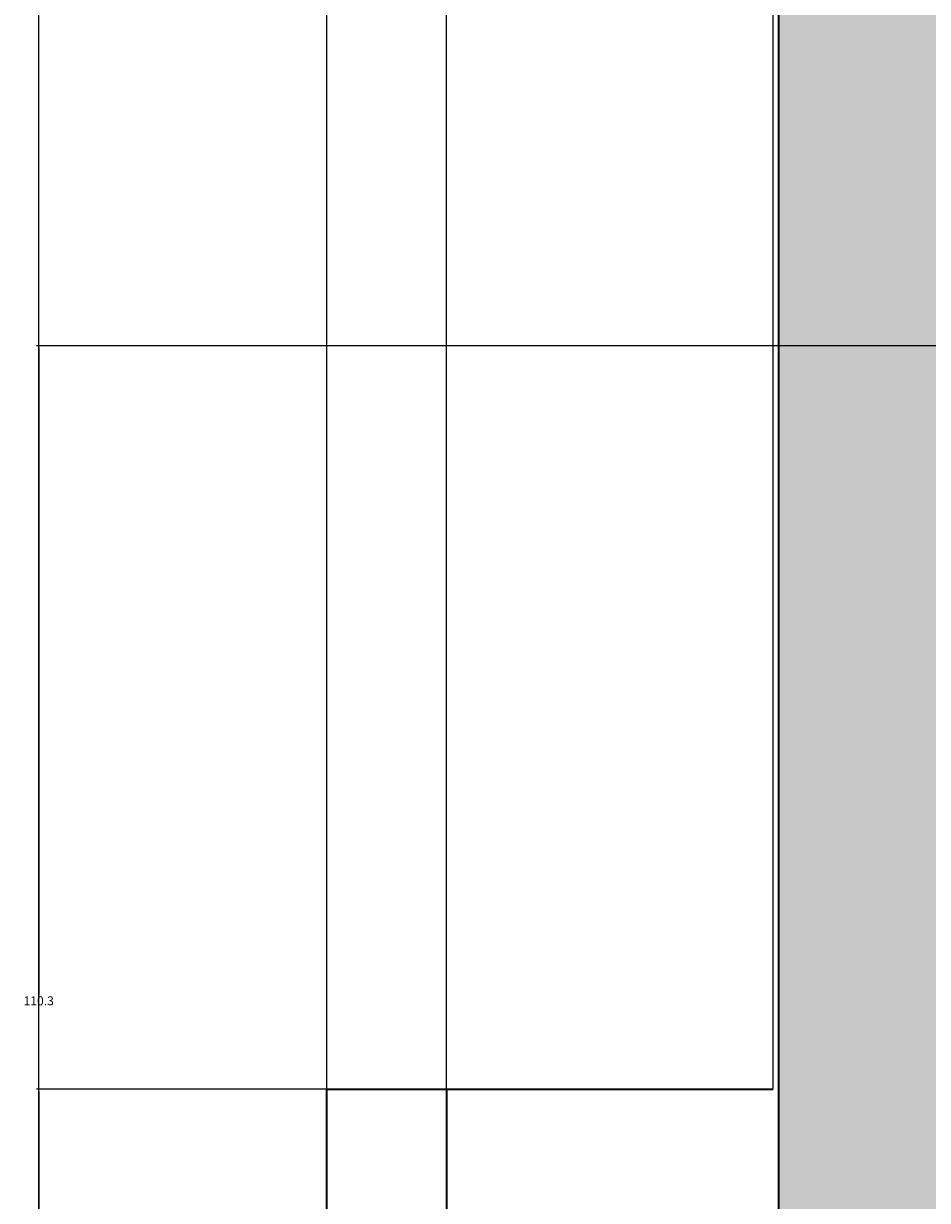
# Model space of a CAD drawing. Units: inches. Extents: x 62 to 566, y 66 to 528.
# Tile 2 of 20: x 62 to 138, y 165 to 264. Entities that reach past the tile are written whole.
import ezdxf

# ---------------------------------------------------------------- set-up
doc = ezdxf.new("R2010")
doc.units = ezdxf.units.IN
doc.header["$MEASUREMENT"] = 0
for name, color, linetype, lineweight in [('A-ANNO-DIMS', 2, 'Continuous', 18), ('A-ELEV', 7, 'Continuous', 35), ('A-WALL-PATT', 8, 'Continuous', 13)]:
    doc.layers.add(name, color=color, linetype=linetype, lineweight=lineweight)
doc.styles.get("Standard").update_dxf_attribs({"font": 'arial.ttf'})
doc.dimstyles.get("Standard").update_dxf_attribs({"dimtxt": 0.75, "dimasz": 0.18, "dimexe": 0.18, "dimexo": 0.0625, "dimgap": 0.09, "dimtad": 0, "dimtih": 1, "dimtoh": 1, "dimdec": 4, "dimzin": 0, "dimdsep": 46, "dimlunit": 4, "dimtxsty": 'Standard', "dimcen": 0.09, "dimadec": 0, "dimazin": 0, "dimtfac": 1, "dimtdec": 4, "dimtofl": 0, "dimtmove": 0, "dimatfit": 3, "dimfxl": 1, "dimtolj": 1, "dimtzin": 0, "dimarcsym": 0})

# ---------------------------------------------------------------- blocks, each defined once
blk = doc.blocks.new('*D8')
at = {"layer": 'A-ANNO-DIMS', "color": 0, "lineweight": -2, "transparency": 16777216}
for p, q in [((284.202, 271.35), (284.202, 65.939)), ((125.942, 126.306), (125.942, 65.939)), ((126.122, 66.119), (203.461, 66.119)), ((284.022, 66.119), (206.683, 66.119))]:
    blk.add_line(p, q, dxfattribs=at)
at = {"layer": 'A-ANNO-DIMS', "color": 0, "transparency": 16777216}
for points in [[(126.122, 66.149), (126.122, 66.089), (125.942, 66.119)], [(284.022, 66.149), (284.022, 66.089), (284.202, 66.119)]]:
    blk.add_solid(points, dxfattribs=at)
at = {"layer": 'Defpoints', "color": 0, "transparency": 16777216}
for p in [(284.202, 271.413), (125.942, 126.369), (284.202, 66.119)]:
    blk.add_point(p, dxfattribs=at)
at = {"layer": 'A-ANNO-DIMS', "color": 0, "transparency": 16777216, "insert": (205.072, 66.119), "char_height": 0.75, "attachment_point": 5}
blk.add_mtext('\\A1;158.26', dxfattribs=at)
blk = doc.blocks.new('*D14')
at = {"layer": 'A-ANNO-DIMS', "color": 0, "lineweight": -2, "transparency": 16777216}
for p, q in [((87.896, 174.128), (87.896, 527.472)), ((88.076, 527.292), (91.611, 527.292)), ((97.787, 527.292), (94.252, 527.292)), ((97.967, 174.128), (97.967, 527.472))]:
    blk.add_line(p, q, dxfattribs=at)
at = {"layer": 'A-ANNO-DIMS', "color": 0, "transparency": 16777216}
for points in [[(88.076, 527.322), (88.076, 527.262), (87.896, 527.292)], [(97.787, 527.322), (97.787, 527.262), (97.967, 527.292)]]:
    blk.add_solid(points, dxfattribs=at)
at = {"layer": 'Defpoints', "color": 0, "transparency": 16777216}
for p in [(97.967, 527.292), (87.896, 174.066), (97.967, 174.066)]:
    blk.add_point(p, dxfattribs=at)
at = {"layer": 'A-ANNO-DIMS', "color": 0, "transparency": 16777216, "insert": (92.932, 527.292), "char_height": 0.75, "attachment_point": 5}
blk.add_mtext('\\A1;10.07', dxfattribs=at)
blk = doc.blocks.new('*D15')
at = {"layer": 'A-ANNO-DIMS', "color": 0, "lineweight": -2, "transparency": 16777216}
for p, q in [((97.967, 174.128), (97.967, 527.472)), ((98.147, 527.292), (110.642, 527.292)), ((125.285, 527.292), (112.789, 527.292)), ((125.465, 174.128), (125.465, 527.472))]:
    blk.add_line(p, q, dxfattribs=at)
at = {"layer": 'A-ANNO-DIMS', "color": 0, "transparency": 16777216}
for points in [[(98.147, 527.322), (98.147, 527.262), (97.967, 527.292)], [(125.285, 527.322), (125.285, 527.262), (125.465, 527.292)]]:
    blk.add_solid(points, dxfattribs=at)
at = {"layer": 'Defpoints', "color": 0, "transparency": 16777216}
for p in [(125.465, 527.292), (97.967, 174.066), (125.465, 174.066)]:
    blk.add_point(p, dxfattribs=at)
at = {"layer": 'A-ANNO-DIMS', "color": 0, "transparency": 16777216, "insert": (111.716, 527.292), "char_height": 0.75, "attachment_point": 5}
blk.add_mtext('\\A1;27.5', dxfattribs=at)
blk = doc.blocks.new('*D17')
at = {"layer": 'A-ANNO-DIMS', "color": 0, "lineweight": -2, "transparency": 16777216}
for p, q in [((87.833694, 174.065908), (63.466194, 174.065908)), ((63.646194, 173.885908), (63.646194, 150.682257)), ((63.646194, 126.548606), (63.646194, 149.752257)), ((87.833694, 126.368606), (63.466194, 126.368606))]:
    blk.add_line(p, q, dxfattribs=at)
at = {"layer": 'A-ANNO-DIMS', "color": 0, "transparency": 16777216}
for points in [[(63.616194, 173.885908), (63.676194, 173.885908), (63.646194, 174.065908)], [(63.616194, 126.548606), (63.676194, 126.548606), (63.646194, 126.368606)]]:
    blk.add_solid(points, dxfattribs=at)
at = {"layer": 'Defpoints', "color": 0, "transparency": 16777216}
for p in [(63.646194, 174.065908), (87.896194, 174.065908), (87.896194, 126.368606)]:
    blk.add_point(p, dxfattribs=at)
at = {"layer": 'A-ANNO-DIMS', "color": 0, "transparency": 16777216, "insert": (63.646194, 150.217257), "char_height": 0.75, "attachment_point": 5}
blk.add_mtext('\\A1;47.7', dxfattribs=at)
blk = doc.blocks.new('*D18')
at = {"layer": 'A-ANNO-DIMS', "color": 0, "lineweight": -2, "transparency": 16777216}
for p, q in [((120.343, 503.042), (63.466, 503.042)), ((63.646, 502.862), (63.646, 339.027)), ((63.646, 174.246), (63.646, 338.081)), ((87.834, 174.066), (63.466, 174.066))]:
    blk.add_line(p, q, dxfattribs=at)
at = {"layer": 'A-ANNO-DIMS', "color": 0, "transparency": 16777216}
for points in [[(63.616, 502.862), (63.676, 502.862), (63.646, 503.042)], [(63.616, 174.246), (63.676, 174.246), (63.646, 174.066)]]:
    blk.add_solid(points, dxfattribs=at)
at = {"layer": 'Defpoints', "color": 0, "transparency": 16777216}
for p in [(63.646, 503.042), (120.406, 503.042), (87.896, 174.066)]:
    blk.add_point(p, dxfattribs=at)
at = {"layer": 'A-ANNO-DIMS', "color": 0, "transparency": 16777216, "insert": (63.646, 338.554), "char_height": 0.75, "attachment_point": 5}
blk.add_mtext('\\A1;329', dxfattribs=at)
blk = doc.blocks.new('*D35')
at = {"layer": 'A-ANNO-DIMS', "color": 0, "lineweight": -2, "transparency": 16777216}
for p, q in [((125.942, 461.98), (125.942, 65.939)), ((142.385, 445.044), (142.385, 65.939)), ((126.122, 66.119), (132.552, 66.119)), ((142.205, 66.119), (135.775, 66.119))]:
    blk.add_line(p, q, dxfattribs=at)
at = {"layer": 'A-ANNO-DIMS', "color": 0, "transparency": 16777216}
for points in [[(126.122, 66.149), (126.122, 66.089), (125.942, 66.119)], [(142.205, 66.149), (142.205, 66.089), (142.385, 66.119)]]:
    blk.add_solid(points, dxfattribs=at)
at = {"layer": 'Defpoints', "color": 0, "transparency": 16777216}
for p in [(125.942, 462.042), (142.385, 445.106), (142.385, 66.119)]:
    blk.add_point(p, dxfattribs=at)
at = {"layer": 'A-ANNO-DIMS', "color": 0, "transparency": 16777216, "insert": (134.163, 66.119), "char_height": 0.75, "attachment_point": 5}
blk.add_mtext('\\A1;16.443', dxfattribs=at)
blk = doc.blocks.new('*D73')
at = {"layer": 'A-ANNO-DIMS', "color": 0, "lineweight": -2, "transparency": 16777216}
for p, q in [((316.148, 236.662), (63.466, 236.662)), ((63.646, 236.482), (63.646, 181.988)), ((63.646, 126.549), (63.646, 181.042)), ((316.148, 126.369), (63.466, 126.369))]:
    blk.add_line(p, q, dxfattribs=at)
at = {"layer": 'A-ANNO-DIMS', "color": 0, "transparency": 16777216}
for points in [[(63.616, 236.482), (63.676, 236.482), (63.646, 236.662)], [(63.616, 126.549), (63.676, 126.549), (63.646, 126.369)]]:
    blk.add_solid(points, dxfattribs=at)
at = {"layer": 'Defpoints', "color": 0, "transparency": 16777216}
for p in [(63.646, 236.662), (316.21, 236.662), (316.21, 126.369)]:
    blk.add_point(p, dxfattribs=at)
at = {"layer": 'A-ANNO-DIMS', "color": 0, "transparency": 16777216, "insert": (63.646, 181.515), "char_height": 0.75, "attachment_point": 5}
blk.add_mtext('\\A1;110.3', dxfattribs=at)

msp = doc.modelspace()

# ---------------------------------------------------------------- hatches: boundary and pattern name
at = {"layer": 'A-WALL-PATT'}
h = msp.add_hatch(color=256, dxfattribs=at)
h.dxf.hatch_style = 1
h.paths.add_polyline_path([(416.0836, 462.0423), (125.9418, 462.0423), (125.9418, 414.3686), (125.9418, 270.3686), (125.9418, 126.3686), (142.3851, 126.3686), (142.3851, 270.3686), (142.3851, 414.3686), (142.3851, 445.1064), (284.2021, 445.1064), (416.0836, 445.1064)])
h.paths.add_polyline_path([(435.3945, 503.0423), (426.3652, 503.0423), (120.4058, 503.0423), (120.4058, 501.0423), (125.9418, 501.0423), (416.0836, 501.0423), (426.3652, 501.0423), (430.6938, 501.0423), (435.3945, 501.0423)])
h.paths.add_polyline_path([(439.6878, 352.4848), (392.4793, 352.4848), (392.4793, 307.4128), (217.2752, 307.4128), (217.2752, 295.4098), (217.2752, 271.4128), (272.0586, 271.4128), (439.6878, 271.4128)])
h.paths.add_polyline_path([(248.0143, 297.1682), (255.6783, 297.1682), (255.6783, 280.0423), (248.0143, 280.0423)], flags=16)
h.paths.add_polyline_path([(235.4641, 280.0423), (227.8001, 280.0423), (227.8001, 297.1682), (235.4641, 297.1682)], flags=16)
h.paths.add_polyline_path([(270.4427, 297.1682), (278.1067, 297.1682), (278.1067, 280.0423), (270.4427, 280.0423)], flags=16)
h.paths.add_polyline_path([(296.3755, 297.1682), (304.0395, 297.1682), (304.0395, 280.0423), (296.3755, 280.0423)], flags=16)
h.paths.add_polyline_path([(319.2543, 297.1682), (326.9183, 297.1682), (326.9183, 280.0423), (319.2543, 280.0423)], flags=16)
h.paths.add_polyline_path([(341.2622, 297.1682), (348.9262, 297.1682), (348.9262, 280.0423), (341.2622, 280.0423)], flags=16)
h.paths.add_polyline_path([(389.2857, 298.3985), (433.8102, 298.3985), (433.8102, 294.9497), (389.2857, 294.9497)], flags=16)
h.paths.add_polyline_path([(389.2857, 291.6038), (433.8102, 291.6038), (433.8102, 288.155), (389.2857, 288.155)], flags=16)
h.paths.add_polyline_path([(389.2857, 284.9607), (433.8102, 284.9607), (433.8102, 281.5119), (389.2857, 281.5119)], flags=16)
h.paths.add_polyline_path([(403.5849, 311.4736), (403.5849, 317.4388), (433.1636, 317.4388), (433.1636, 311.4736)], flags=16)
h.paths.add_polyline_path([(403.5849, 323.1329), (403.5849, 329.0982), (433.1636, 329.0982), (433.1636, 323.1329)], flags=16)
h.paths.add_polyline_path([(403.5849, 334.5211), (403.5849, 340.4863), (433.1636, 340.4863), (433.1636, 334.5211)], flags=16)
h.paths.add_polyline_path([(272.0586, 160.3545), (217.2752, 160.3545), (217.2752, 129.0504), (217.2752, 126.3686), (272.0586, 126.3686)], flags=17)
h.paths.add_polyline_path([(220.5897, 149.5749), (220.5897, 152.296), (267.7931, 152.296), (267.7931, 149.5749)], flags=16)
h.paths.add_polyline_path([(267.7931, 146.6724), (267.7931, 143.9513), (220.5897, 143.9513), (220.5897, 146.6724)], flags=16)
h.paths.add_polyline_path([(220.5897, 155.3799), (220.5897, 158.101), (267.7931, 158.101), (267.7931, 155.3799)], flags=16)
h.paths.add_polyline_path([(267.7931, 140.686), (267.7931, 137.9649), (220.5897, 137.9649), (220.5897, 140.686)], flags=16)
h.paths.add_polyline_path([(267.7931, 135.516), (267.7931, 132.7949), (220.5897, 132.7949), (220.5897, 135.516)], flags=16)

# ---------------------------------------------------------------- linework, layer by layer
at = {"layer": 'A-ELEV'}
for p, q in [((125.9418, 126.3686), (125.9418, 270.3686)), ((87.8962, 126.3686), (87.8962, 174.0659)), ((87.8962, 174.0659), (97.967, 174.0659)), ((97.967, 174.0659), (97.967, 126.3686)), ((97.967, 174.0659), (125.4645, 174.0659))]:
    msp.add_line(p, q, dxfattribs=at)

# ---------------------------------------------------------------- dimensions: what is measured, and where the dimension line sits
at = {"layer": 'A-ANNO-DIMS'}
for base, p1, p2, override, picture, middle in [((97.967, 527.2923), (87.8962, 174.0659), (97.967, 174.0659), {"dimdec": 2, "dimlfac": 1, "dimrnd": 0, "dimzin": 0, "dimdsep": 46, "dimlunit": 2}, '*D14', (92.9316, 527.2923)), ((125.4645, 527.2923), (97.967, 174.0659), (125.4645, 174.0659), {"dimdec": 1, "dimlfac": 1, "dimrnd": 0, "dimzin": 0, "dimdsep": 46, "dimlunit": 2}, '*D15', (111.7157, 527.2923)), ((142.3851, 66.1186), (125.9418, 462.0423), (142.3851, 445.1064), {"dimdec": 3, "dimlfac": 1, "dimrnd": 0, "dimzin": 0, "dimdsep": 46, "dimlunit": 2}, '*D35', (134.1634, 66.1186)), ((284.2021, 66.1186), (125.9418, 126.3686), (284.2021, 271.4128), {"dimdec": 2, "dimlfac": 1, "dimrnd": 0, "dimzin": 0, "dimdsep": 46, "dimlunit": 2}, '*D8', (205.0719, 66.1186))]:
    dim = msp.add_linear_dim(base=base, p1=p1, p2=p2, dimstyle='Standard', override=override, dxfattribs=at)
    dim.commit()
    dim.dimension.update_dxf_attribs({"geometry": picture, "text_midpoint": middle})
for base, p1, p2, override, picture, middle in [((63.6462, 503.0423), (87.8962, 174.0659), (120.4058, 503.0423), {"dimdec": 0, "dimlfac": 1, "dimrnd": 0, "dimzin": 0, "dimdsep": 46, "dimlunit": 2}, '*D18', (63.6462, 338.5541)), ((63.6462, 236.6618), (316.2101, 126.3686), (316.2101, 236.6618), {"dimdec": 1, "dimlfac": 1, "dimrnd": 0, "dimzin": 0, "dimdsep": 46, "dimlunit": 2}, '*D73', (63.6462, 181.5152)), ((63.6462, 174.0659), (87.8962, 126.3686), (87.8962, 174.0659), {"dimdec": 1, "dimlfac": 1, "dimrnd": 0, "dimzin": 0, "dimdsep": 46, "dimlunit": 2}, '*D17', (63.6462, 150.2173))]:
    dim = msp.add_linear_dim(base=base, p1=p1, p2=p2, angle=90, dimstyle='Standard', override=override, dxfattribs=at)
    dim.commit()
    dim.dimension.update_dxf_attribs({"geometry": picture, "text_midpoint": middle})

doc.saveas('drawing.dxf')
